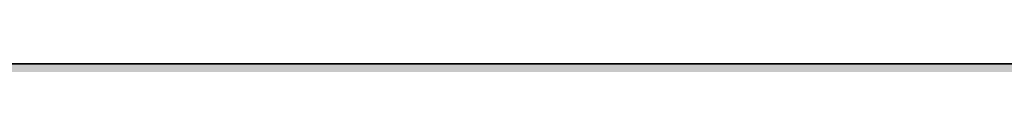
# Model space of a CAD drawing. Units: inches. Extents: x 2091 to 2899, y 967 to 2217.
# Tile 100 of 256: x 2252.3817 to 2252.951, y 1099.9191 to 1099.9191. Entities that reach past the tile are written whole.
import ezdxf

# ---------------------------------------------------------------- set-up
doc = ezdxf.new("R2010")
doc.units = ezdxf.units.IN
doc.layers.add('A-WALL-PATT', color=141, linetype='Continuous', lineweight=13, true_color=0xadddf7)
doc.layers.add('L-SITE-WALL', color=7, linetype='Continuous', lineweight=35)

msp = doc.modelspace()

# ---------------------------------------------------------------- hatches: boundary and pattern name
at = {"layer": 'A-WALL-PATT'}
h = msp.add_hatch(color=256, dxfattribs=at)
h.dxf.hatch_style = 1
h.paths.add_polyline_path([(2212.1436, 1941.41906), (2387.6436, 1941.41906), (2387.6436, 1824.41906), (2392.1436, 1824.41906), (2392.1436, 1941.41906), (2609.6436, 1941.41906), (2609.6436, 1825.91906), (2614.1436, 1825.91906), (2614.1436, 1941.41906), (2794.1436, 1941.41906), (2794.1436, 1928.76217), (2803.1436, 1928.76217), (2803.1436, 2050.91906), (2203.1436, 2050.91906), (2203.1436, 1900.75786), (2212.1436, 1900.75786)])
h.paths.add_polyline_path([(2212.1436, 1945.91906), (2212.1436, 2041.91906), (2794.1436, 2041.91906), (2794.1436, 1945.91906), (2402.24824, 1945.91906), (2401.10243, 1945.77583), (2398.70243, 1945.77583)], flags=16)
h.paths.add_polyline_path([(2230.22986, 1948.06279), (2227.34986, 1949.50279), (2225.90986, 1951.90279), (2223.98986, 1952.86279), (2223.02986, 1955.26279), (2222.06986, 1959.58279), (2222.06986, 1963.42279), (2223.02986, 1965.66279), (2223.98986, 1965.34279), (2225.58591, 1963.86075), (2226.91153, 1964.95726), (2226.94886, 1965.93879), (2227.77832, 1966.95214), (2228.19992, 1968.8787), (2230.70986, 1964.86279), (2233.58986, 1966.30279), (2233.60731, 1966.33187), (2233.77266, 1964.9382), (2234.6338, 1963.67647), (2235.02986, 1963.90279), (2236.28203, 1965.57236), (2235.98986, 1962.94279), (2237.95451, 1957.54), (2238.38986, 1957.90279), (2239.21586, 1960.30579), (2238.65457, 1966.38496), (2238.69279, 1966.43807), (2238.84058, 1967.49971), (2238.78029, 1967.68749), (2238.88054, 1967.78676), (2238.66686, 1966.25179), (2239.21586, 1960.30579), (2238.38986, 1957.90279), (2236.94986, 1956.70279), (2234.54986, 1949.98279)], flags=0)
h.paths.add_polyline_path([(2278.01197, 1948.06279), (2276.49643, 1947.87335), (2275.84983, 1947.68861), (2274.65197, 1947.10279)], flags=0)
h.paths.add_polyline_path([(2269.85197, 1955.74279), (2268.27618, 1956.62933), (2270.8673, 1956.3484), (2269.37197, 1958.14279), (2268.71496, 1959.19233), (2270.56983, 1958.72861), (2268.58073, 1961.90609), (2270.81197, 1960.89188), (2270.81197, 1963.42279), (2271.39331, 1964.77926), (2270.29176, 1966.1562), (2271.77197, 1965.66279), (2272.14139, 1966.52476), (2273.92983, 1965.92861), (2275.63039, 1968.0543), (2276.33194, 1966.72186), (2276.52043, 1966.95214), (2276.94203, 1968.8787), (2277.73429, 1967.61108), (2278.13989, 1969.46452), (2279.65912, 1967.03374), (2280.41197, 1966.78279), (2280.9493, 1967.58879), (2281.60983, 1967.36861), (2282.13327, 1968.15376), (2282.34924, 1966.33344), (2282.34985, 1966.33259), (2283.40755, 1968.09542), (2283.71263, 1965.52402), (2284.32022, 1964.63379), (2284.51181, 1964.88924), (2284.23497, 1965.70479), (2284.50047, 1967.31896), (2284.90794, 1965.41742), (2285.39631, 1966.06858), (2285.43283, 1966.29061), (2285.47334, 1966.17128), (2286.35392, 1967.34539), (2286.22201, 1966.15817), (2287.66349, 1968.08015), (2287.71397, 1968.44279), (2288.4816, 1969.01668), (2288.57399, 1968.7289), (2288.91746, 1969.06904), (2288.60683, 1966.83761), (2288.92873, 1963.35131), (2288.93497, 1963.35679), (2288.92973, 1963.34042), (2289.01528, 1962.41387), (2290.11122, 1963.87513), (2290.13283, 1963.94261), (2290.21767, 1964.01706), (2290.11122, 1963.87513), (2289.15583, 1960.89161), (2288.59404, 1959.25723), (2288.57197, 1959.10279), (2289.53197, 1960.54279), (2290.01197, 1962.46279), (2290.19184, 1962.64266), (2289.76983, 1959.68861), (2286.88983, 1957.28861), (2284.48983, 1950.56861), (2283.31466, 1950.04631), (2283.29197, 1949.98279), (2280.29006, 1948.64861), (2281.12983, 1948.64861), (2282.56983, 1948.16861), (2283.20473, 1948.06279), (2278.97197, 1948.06279), (2276.09197, 1949.50279), (2274.65197, 1951.90279), (2272.73197, 1952.86279)], flags=0)
h.paths.add_polyline_path([(2271.15887, 1958.02177), (2272.96983, 1955.84861), (2272.00983, 1960.16861), (2272.00983, 1964.00861), (2272.62443, 1965.44266), (2274.32802, 1963.86075), (2275.65365, 1964.95726), (2275.63774, 1964.53909), (2277.41223, 1966.00689), (2277.03297, 1965.15679), (2276.82992, 1964.9756), (2276.76601, 1963.29501), (2277.44964, 1962.66022), (2279.45197, 1964.86279), (2282.33197, 1966.30279), (2283.52983, 1966.88861), (2283.29451, 1966.77095), (2283.91299, 1963.8847), (2284.89925, 1964.44827), (2284.73197, 1962.94279), (2286.69662, 1957.54), (2287.13197, 1957.90279), (2287.54191, 1959.09539), (2287.7794, 1958.44231), (2285.68274, 1956.6951), (2285.8765, 1959.79534), (2284.73197, 1962.94279), (2284.89925, 1964.44827), (2283.91299, 1963.8847), (2284.22383, 1962.43412), (2283.42436, 1963.60548), (2281.60983, 1962.56861), (2281.12983, 1960.16861), (2282.08983, 1956.32861), (2283.04983, 1952.96861), (2282.56983, 1950.56861), (2280.16983, 1948.64861), (2279.88332, 1948.79187), (2278.97197, 1948.06279), (2278.97197, 1949.02279), (2278.67231, 1949.39737), (2277.28983, 1950.08861), (2275.84983, 1952.48861), (2273.92983, 1953.44861), (2272.48983, 1954.88861), (2271.92165, 1954.88861), (2271.77197, 1955.26279)], flags=0)
h.paths.add_polyline_path([(2311.99415, 1955.74279), (2312.06272, 1955.67422), (2312.0551, 1955.7085)], flags=0)
h.paths.add_polyline_path([(2331.95615, 1963.95179), (2333.39615, 1965.39179), (2331.07715, 1963.35679), (2330.9986, 1963.11152)], flags=0)
h.paths.add_polyline_path([(2310.55415, 1954.30279), (2307.03981, 1956.27994), (2310.7629, 1955.87628), (2312.47415, 1953.82279), (2313.43415, 1951.42279), (2315.35415, 1950.46279), (2316.79415, 1948.06279), (2317.46615, 1947.72679), (2319.36869, 1947.96461), (2317.75415, 1949.98279), (2317.56953, 1950.61048), (2316.79415, 1951.90279), (2314.87415, 1952.86279), (2313.91415, 1955.26279), (2311.51415, 1958.14279), (2309.37549, 1961.55917), (2311.51415, 1960.33708), (2311.51415, 1961.98279), (2310.60467, 1963.11963), (2311.72661, 1962.47853), (2312.41833, 1964.09256), (2312.25596, 1964.29552), (2313.19415, 1963.98279), (2313.91415, 1965.66279), (2314.64678, 1965.41858), (2315.35415, 1966.30279), (2316.79415, 1967.74279), (2316.15744, 1966.9469), (2317.03411, 1965.28186), (2317.2226, 1965.51214), (2317.77705, 1968.04577), (2318.47411, 1966.72186), (2318.6626, 1966.95214), (2319.0842, 1968.8787), (2321.20705, 1965.48215), (2322.16142, 1966.9137), (2322.55415, 1966.78279), (2322.78599, 1967.13056), (2322.88165, 1966.32429), (2323.31204, 1965.72174), (2323.65129, 1965.89136), (2324.3965, 1967.13338), (2324.65694, 1964.9382), (2324.97199, 1964.47661), (2325.38728, 1967.0015), (2325.94081, 1964.41835), (2327.22893, 1966.13584), (2327.16632, 1965.57236), (2328.05914, 1966.76278), (2328.22458, 1966.24749), (2329.66797, 1967.67691), (2329.66458, 1967.68749), (2329.76482, 1967.78676), (2329.55115, 1966.25179), (2330.10015, 1960.30579), (2329.33281, 1958.07347), (2329.31306, 1957.93523), (2329.63415, 1958.20279), (2330.23415, 1959.10279), (2330.71415, 1961.02279), (2331.03415, 1961.34279), (2330.71415, 1959.10279), (2329.63415, 1958.20279), (2329.27415, 1957.66279), (2327.71211, 1956.3611), (2325.43415, 1949.98279), (2324.33377, 1949.49374), (2323.99415, 1948.54279), (2319.67415, 1946.62279), (2316.79415, 1948.06279), (2315.35415, 1950.46279), (2313.43415, 1951.42279)], flags=0)
h.paths.add_polyline_path([(2321.33568, 1947.95202), (2321.11415, 1948.06279), (2321.11415, 1949.02279), (2319.19415, 1951.42279), (2316.79415, 1959.58279), (2316.66324, 1959.58279), (2315.35415, 1958.14279), (2314.39415, 1958.14279), (2313.1483, 1958.70908), (2312.95415, 1959.58279), (2312.95415, 1960.89188), (2315.83415, 1959.58279), (2316.66324, 1959.58279), (2317.31471, 1960.29941), (2315.0302, 1962.42075), (2316.35582, 1963.51726), (2316.37234, 1963.95162), (2316.4702, 1963.86075), (2317.79582, 1964.95726), (2317.75522, 1963.88969), (2319.17515, 1965.15679), (2319.49841, 1965.88137), (2321.11415, 1965.34279), (2323.23589, 1962.37236), (2325.68635, 1963.77262), (2325.54279, 1962.48058), (2325.19878, 1963.49401), (2324.47851, 1963.08243), (2324.92601, 1960.99412), (2324.07809, 1962.23647), (2322.41479, 1961.28602), (2322.07415, 1959.58279), (2323.03415, 1955.74279), (2323.99415, 1952.38279), (2323.51415, 1949.98279), (2322.14272, 1948.88565), (2322.07415, 1948.54279)], flags=0)
h.paths.add_polyline_path([(2320.20748, 1963.33746), (2320.15415, 1963.42279), (2320.39415, 1963.54279)], flags=0)
h.paths.add_polyline_path([(2353.85053, 1965.8105), (2354.03053, 1965.7505), (2354.33053, 1966.4505), (2354.33053, 1966.9305)], flags=0)
h.paths.add_polyline_path([(2359.02058, 1969.02641), (2359.09838, 1968.90193), (2359.23353, 1969.5195), (2359.23353, 1969.9995)], flags=0)
h.paths.add_polyline_path([(2358.25669, 1966.68167), (2357.9836, 1966.34803), (2358.21127, 1966.14617), (2358.41049, 1966.38957)], flags=0)
h.paths.add_polyline_path([(2357.76847, 1966.05878), (2357.7322, 1965.10497), (2357.75105, 1965.12056), (2357.76953, 1965.6065), (2357.76953, 1966.05784)], flags=0)
h.paths.add_polyline_path([(2359.11153, 1965.3045), (2359.11153, 1964.8245), (2359.84453, 1966.4675), (2359.84453, 1966.9475)], flags=0)
h.paths.add_polyline_path([(2360.22368, 1966.62145), (2360.69853, 1969.3625), (2360.69853, 1969.8425), (2360.21053, 1967.0255), (2360.21053, 1966.6425)], flags=0)
h.paths.add_polyline_path([(2363.45053, 1967.8905), (2363.45053, 1968.3705), (2362.49053, 1966.9305), (2362.65604, 1966.69878)], flags=0)
h.paths.add_polyline_path([(2364.47552, 1966.07883), (2365.85053, 1968.3705), (2365.85053, 1968.8505), (2364.42798, 1966.47958)], flags=0)
h.paths.add_polyline_path([(2366.31353, 1965.8525), (2366.36671, 1965.69583), (2366.80253, 1968.3455), (2366.80253, 1968.8255)], flags=0)
h.paths.add_polyline_path([(2367.16531, 1965.80354), (2367.29053, 1966.9305), (2367.29053, 1967.4105), (2367.1027, 1965.72007)], flags=0)
h.paths.add_polyline_path([(2370.03653, 1959.9735), (2371.01353, 1963.0245), (2371.01353, 1963.5045), (2370.03653, 1960.4535)], flags=0)
h.paths.add_polyline_path([(2371.61053, 1960.2105), (2372.57053, 1961.6505), (2372.57053, 1962.1305), (2371.80253, 1960.9785)], flags=0)
h.paths.add_polyline_path([(2350.87367, 1956.00509), (2351.93053, 1955.8905), (2354.49053, 1953.3305), (2353.85053, 1954.9305), (2351.45053, 1957.8105), (2347.93553, 1963.4255), (2347.93553, 1963.9055), (2351.45053, 1958.2905), (2353.70507, 1955.58505), (2352.89053, 1959.2505), (2352.89053, 1959.7305), (2352.89053, 1961.92479), (2356.73053, 1959.7305), (2358.45447, 1961.62684), (2354.81053, 1965.0105), (2355.03086, 1965.28591), (2358.69109, 1961.88712), (2361.53053, 1965.0105), (2364.3765, 1966.43348), (2364.52439, 1965.18691), (2365.45447, 1963.82418), (2365.88107, 1964.06795), (2365.37053, 1966.4505), (2365.37053, 1966.9305), (2366.81053, 1960.2105), (2366.81053, 1959.7305), (2366.38871, 1952.98141), (2367.77053, 1956.8505), (2368.64123, 1957.57608), (2366.81053, 1962.6105), (2366.81053, 1963.0905), (2368.77518, 1957.68771), (2369.21053, 1958.0505), (2370.00159, 1960.35187), (2369.47523, 1966.05267), (2369.51346, 1966.10578), (2369.51417, 1966.11091), (2369.47523, 1966.53267), (2369.51346, 1966.58578), (2369.61463, 1967.31259), (2369.18253, 1968.6585), (2369.18253, 1969.1385), (2369.60096, 1967.83519), (2369.7012, 1967.93447), (2369.71795, 1968.05474), (2370.14518, 1968.37414), (2369.77871, 1968.01122), (2369.7012, 1967.45447), (2370.46816, 1968.214), (2369.67494, 1967.26577), (2369.51417, 1966.11091), (2370.03653, 1960.4535), (2370.03653, 1959.9735), (2369.44176, 1958.24319), (2370.65053, 1959.2505), (2371.04582, 1962.01756), (2371.13053, 1962.1305), (2370.65053, 1958.7705), (2367.77053, 1956.3705), (2365.37053, 1949.6505), (2362.0791, 1948.18764), (2363.45053, 1947.7305), (2361.05053, 1947.7305), (2360.09053, 1947.7305), (2357.10386, 1947.35717), (2360.09053, 1948.2105), (2358.17053, 1949.1705), (2356.73053, 1951.5705), (2354.81053, 1952.5305), (2351.93053, 1955.4105)], flags=0)
h.paths.add_polyline_path([(2361.05053, 1948.6905), (2359.13053, 1951.0905), (2356.73053, 1959.2505), (2355.77053, 1959.2505), (2352.89053, 1960.55959), (2352.89053, 1961.44479), (2355.89053, 1959.7305), (2356.73053, 1959.7305), (2356.83719, 1959.36783), (2361.53053, 1964.5305), (2363.24842, 1965.38945), (2364.92531, 1963.0418), (2362.49053, 1961.6505), (2362.06386, 1959.51717), (2362.97053, 1955.8905), (2363.93053, 1952.5305), (2363.93053, 1952.0505), (2363.45053, 1949.6505), (2361.05053, 1947.7305)], flags=0)
h.paths.add_polyline_path([(2359.13053, 1951.5705), (2359.29053, 1951.3705), (2361.05053, 1954.4505), (2361.05053, 1954.9305)], flags=0)
h.paths.add_polyline_path([(2357.21953, 1966.5455), (2356.79253, 1968.8145), (2356.79253, 1969.2945), (2357.21953, 1967.0255)], flags=0)
h.paths.add_polyline_path([(2361.05053, 1954.4505), (2361.53053, 1958.7705), (2361.53053, 1959.2505), (2361.05053, 1954.9305)], flags=0)
h.paths.add_polyline_path([(2402.54829, 1948.48608), (2402.30243, 1948.41583), (2402.59043, 1948.41583)], flags=0)
h.paths.add_polyline_path([(2394.14243, 1956.09583), (2395.68505, 1954.55321), (2396.7205, 1953.97068), (2396.06243, 1955.61583), (2395.24138, 1956.6011), (2395.8789, 1956.44171), (2395.10243, 1959.93583), (2395.10243, 1963.77583), (2396.06243, 1966.01583), (2397.02243, 1965.69583), (2398.61848, 1964.21379), (2399.94411, 1965.3103), (2399.98143, 1966.29183), (2400.81089, 1967.30518), (2401.23249, 1969.23174), (2403.53795, 1965.54301), (2403.94198, 1967.38932), (2404.70243, 1967.13583), (2405.46033, 1966.07478), (2406.62243, 1966.65583), (2406.63988, 1966.68491), (2406.80523, 1965.29124), (2406.92569, 1965.11475), (2407.34243, 1964.97583), (2407.87433, 1965.77367), (2408.1691, 1964.39805), (2409.31461, 1965.9254), (2409.21746, 1965.05105), (2409.44523, 1963.13124), (2410.30637, 1961.86951), (2410.70243, 1962.09583), (2411.44227, 1963.08228), (2411.16543, 1963.89783), (2411.61643, 1966.63976), (2411.72536, 1966.79111), (2411.87315, 1967.85275), (2411.81286, 1968.04053), (2411.91311, 1968.1398), (2411.69943, 1966.60483), (2412.24843, 1960.65883), (2413.22543, 1963.70983), (2414.3779, 1964.72116), (2414.51315, 1965.69275), (2414.45286, 1965.88053), (2414.55311, 1965.9798), (2414.3779, 1964.72116), (2414.51982, 1964.8457), (2414.36536, 1964.63111), (2414.33943, 1964.44483), (2414.88843, 1958.49883), (2414.06243, 1956.09583), (2412.62243, 1954.89583), (2410.17137, 1948.03285), (2410.01672, 1948.0844), (2405.90243, 1946.25583), (2405.90243, 1947.21583), (2405.20425, 1948.08856), (2404.22243, 1948.41583), (2403.26243, 1948.41583), (2400.38243, 1949.85583), (2399.66243, 1951.05583), (2397.98243, 1952.73583), (2397.02243, 1953.21583), (2395.68505, 1954.55321), (2392.65678, 1956.25691)], flags=0)
h.paths.add_polyline_path([(2409.08565, 1964.40744), (2409.13036, 1964.27572), (2409.26243, 1964.49583)], flags=0)
h.paths.add_polyline_path([(2397.74243, 1961.61583), (2398.70243, 1963.85583), (2399.66243, 1963.53583), (2401.42656, 1965.74099), (2401.79142, 1966.5588), (2402.07143, 1965.07083), (2402.83551, 1964.39337), (2403.2624, 1964.9149), (2403.33812, 1964.77109), (2402.61552, 1963.97622), (2402.49861, 1960.90224), (2403.543, 1959.93245), (2404.4132, 1960.88968), (2404.70243, 1962.33583), (2407.91635, 1964.17235), (2409.52021, 1961.92694), (2410.98708, 1957.89304), (2411.42243, 1958.25583), (2412.04796, 1960.07562), (2412.41034, 1959.07909), (2411.67562, 1958.46682), (2411.66243, 1958.25583), (2411.62607, 1958.42553), (2409.98243, 1957.05583), (2407.58243, 1950.33583), (2403.26243, 1948.41583), (2403.26243, 1949.37583), (2401.34243, 1951.77583), (2399.41651, 1958.32398), (2397.74243, 1959.08492), (2397.74243, 1959.97012), (2397.10243, 1960.33583), (2397.74243, 1960.04492)], flags=0)
h.paths.add_polyline_path([(2405.90243, 1952.97583), (2405.95043, 1953.40783), (2406.01672, 1953.17583)], flags=0)
h.paths.add_polyline_path([(2449.81778, 1967.11401), (2449.75232, 1967.13583), (2449.7937, 1967.0779)], flags=0)
h.paths.add_polyline_path([(2451.6977, 1966.61812), (2451.74089, 1966.69012), (2451.69205, 1966.6657)], flags=0)
h.paths.add_polyline_path([(2454.34363, 1965.73757), (2455.75232, 1967.61583), (2455.99232, 1968.09583), (2454.3645, 1965.9254)], flags=0)
h.paths.add_polyline_path([(2457.54732, 1968.86383), (2457.78732, 1969.34383), (2457.05432, 1968.79583), (2457.00762, 1968.46034)], flags=0)
h.paths.add_polyline_path([(2456.92178, 1967.85666), (2456.80224, 1968.22902), (2456.723, 1967.6598)], flags=0)
h.paths.add_polyline_path([(2457.30232, 1967.37683), (2457.54232, 1967.85683), (2456.81032, 1966.83983), (2456.74052, 1966.70022), (2456.74902, 1966.60811)], flags=0)
h.paths.add_polyline_path([(2458.27532, 1963.70983), (2458.15534, 1963.33515), (2460.35432, 1965.26483), (2460.59432, 1965.74483)], flags=0)
h.paths.add_polyline_path([(2458.39232, 1962.81583), (2458.36409, 1962.61819), (2459.59232, 1964.25583), (2459.83232, 1964.73583)], flags=0)
h.paths.add_polyline_path([(2459.35232, 1962.81583), (2459.27232, 1962.49583), (2460.07232, 1963.29583), (2460.31232, 1963.77583)], flags=0)
h.paths.add_polyline_path([(2458.68032, 1960.60783), (2458.63232, 1960.41583), (2459.59232, 1961.85583), (2459.83232, 1962.33583)], flags=0)
h.paths.add_polyline_path([(2437.83817, 1956.24265), (2439.19232, 1956.09583), (2441.35232, 1953.93583), (2440.87232, 1955.13583), (2438.47232, 1958.01583), (2438.07156, 1958.65602), (2438.71232, 1958.49583), (2440.6396, 1956.18311), (2439.91232, 1959.45583), (2439.91232, 1963.29583), (2441.35232, 1966.65583), (2441.59232, 1967.13583), (2441.11232, 1966.01583), (2442.07232, 1965.69583), (2443.98899, 1968.09167), (2444.24132, 1966.75083), (2444.9168, 1966.15192), (2445.67657, 1967.08014), (2446.25532, 1969.72483), (2446.49532, 1970.20483), (2446.28238, 1969.23174), (2447.36267, 1967.50327), (2447.72032, 1969.56783), (2447.96032, 1970.04783), (2447.48548, 1967.30678), (2448.79232, 1965.21583), (2448.47232, 1964.86383), (2448.55232, 1964.73583), (2451.45205, 1966.1857), (2451.61512, 1964.81124), (2452.30792, 1963.79617), (2453.23451, 1964.32565), (2454.07232, 1960.41583), (2453.62869, 1953.31765), (2454.79232, 1956.57583), (2455.03232, 1957.05583), (2455.71884, 1957.62793), (2453.83232, 1962.81583), (2453.94097, 1963.79362), (2453.33532, 1965.57783), (2453.82432, 1968.55083), (2454.06432, 1969.03083), (2453.57532, 1966.05783), (2454.04033, 1964.68792), (2453.83232, 1962.81583), (2455.71884, 1957.62793), (2456.36721, 1958.16824), (2457.05832, 1960.17883), (2457.29832, 1960.65883), (2456.47232, 1958.25583), (2457.71773, 1959.29367), (2457.67232, 1958.97583), (2454.88995, 1956.65719), (2453.61414, 1953.08492), (2453.59232, 1952.73583), (2453.35232, 1952.25583), (2453.3596, 1952.3722), (2452.63232, 1950.33583), (2452.39232, 1949.85583), (2449.20375, 1948.43869), (2450.71232, 1947.93583), (2448.07232, 1947.93583), (2447.11232, 1947.93583), (2444.55232, 1947.61583), (2447.1996, 1948.3722), (2445.19232, 1949.37583), (2443.75232, 1951.77583), (2441.83232, 1952.73583), (2438.95232, 1955.61583)], flags=0)
h.paths.add_polyline_path([(2443.99232, 1959.93583), (2444.04032, 1959.77263), (2444.12155, 1959.86199)], flags=0)
h.paths.add_polyline_path([(2442.91232, 1959.93583), (2443.03232, 1959.93583), (2442.44566, 1960.2025)], flags=0)
h.paths.add_polyline_path([(2444.98294, 1965.01968), (2445.27932, 1965.26483), (2445.51932, 1965.74483), (2444.994, 1965.3103)], flags=0)
h.paths.add_polyline_path([(2446.13332, 1965.02983), (2446.33037, 1965.4715), (2444.97032, 1964.25783), (2444.73032, 1963.77783)], flags=0)
h.paths.add_polyline_path([(2442.79232, 1959.45583), (2443.75232, 1959.45583), (2446.15232, 1951.29583), (2446.41232, 1951.75083), (2446.39232, 1951.77583), (2448.0806, 1954.73032), (2448.55232, 1958.97583), (2441.83232, 1965.21583), (2442.15495, 1965.61911), (2448.79232, 1959.45583), (2448.31232, 1955.13583), (2448.07232, 1954.65583), (2446.41232, 1951.75083), (2448.31232, 1949.37583), (2448.31232, 1948.41583), (2450.54089, 1950.19869), (2450.95232, 1952.25583), (2449.99232, 1955.61583), (2449.03232, 1959.45583), (2449.51232, 1961.85583), (2449.75232, 1962.33583), (2449.6749, 1961.94874), (2452.99451, 1963.84565), (2453.06441, 1963.51941), (2452.88461, 1963.78285), (2449.6749, 1961.94874), (2449.27232, 1959.93583), (2450.23232, 1956.09583), (2451.19232, 1952.73583), (2450.71232, 1950.33583), (2450.47232, 1949.85583), (2448.07232, 1947.93583), (2448.07232, 1948.53583), (2445.43232, 1949.85583), (2443.99232, 1952.25583), (2442.07232, 1953.21583), (2441.11232, 1955.61583), (2440.15232, 1959.93583), (2440.15232, 1960.65583)], flags=0)
h.paths.add_polyline_path([(2456.69232, 1966.98583), (2457.60832, 1968.08083), (2457.84832, 1968.56083), (2456.93232, 1967.46583)], flags=0)
h.paths.add_polyline_path([(2489.89657, 1966.58024), (2489.94295, 1966.18935), (2490.74749, 1967.53025), (2491.31912, 1968.95116)], flags=0)
h.paths.add_polyline_path([(2473.56247, 1956.40713), (2477.13998, 1956.01926), (2476.95533, 1956.24083), (2475.10805, 1957.28011), (2476.34749, 1956.97025), (2475.1869, 1958.82422), (2476.91912, 1958.39116), (2475.41164, 1960.79927), (2477.78749, 1959.71934), (2477.78749, 1962.25025), (2477.6374, 1962.43786), (2477.82255, 1962.33206), (2478.35912, 1963.58406), (2478.35912, 1963.67116), (2477.32435, 1964.96463), (2478.71483, 1964.50114), (2479.31912, 1965.91116), (2480.27912, 1965.59116), (2481.78397, 1967.47221), (2482.11649, 1965.70525), (2482.88056, 1965.02778), (2483.20931, 1965.42941), (2483.22017, 1965.71509), (2483.07594, 1965.98902), (2483.71176, 1966.76581), (2484.13049, 1968.67925), (2484.70212, 1970.10016), (2484.48918, 1969.12707), (2486.5029, 1965.90511), (2487.38749, 1965.61025), (2488.15342, 1966.75914), (2488.71702, 1965.97011), (2489.20009, 1966.21164), (2489.33067, 1965.11099), (2490.3939, 1963.62246), (2490.66077, 1963.77496), (2490.49391, 1964.55364), (2490.92306, 1963.92484), (2491.31912, 1964.15116), (2491.33339, 1964.17018), (2491.21049, 1964.53225), (2491.28176, 1964.96554), (2491.42579, 1964.29338), (2494.07648, 1967.82763), (2494.49792, 1966.51494), (2494.59817, 1966.61422), (2494.68949, 1967.27025), (2495.10675, 1967.5822), (2495.12984, 1967.74807), (2495.06955, 1967.93585), (2495.1698, 1968.03513), (2495.03178, 1967.04363), (2495.75382, 1967.75868), (2494.98205, 1966.68644), (2494.95612, 1966.50016), (2495.47902, 1960.83685), (2495.91049, 1962.18425), (2496.48212, 1963.60516), (2496.07269, 1962.32659), (2496.7689, 1962.93754), (2496.59912, 1962.71116), (2496.11912, 1959.35116), (2496.73287, 1960.27179), (2496.98749, 1961.29025), (2497.55912, 1962.71116), (2497.07912, 1960.79116), (2496.50749, 1959.37025), (2495.54749, 1957.93025), (2492.75884, 1955.60638), (2490.83912, 1950.23116), (2490.26749, 1948.81025), (2485.94749, 1946.89025), (2483.06749, 1948.33025), (2481.62749, 1950.73025), (2479.70749, 1951.69025), (2476.82749, 1954.57025)], flags=0)
h.paths.add_polyline_path([(2485.57697, 1948.31339), (2485.55912, 1948.31116), (2485.57876, 1948.31116)], flags=0)
h.paths.add_polyline_path([(2478.64506, 1954.55116), (2478.10904, 1956.96326), (2479.31912, 1955.51116), (2480.27912, 1953.11116), (2482.19912, 1952.15116), (2483.63912, 1949.75116), (2486.51912, 1948.31116), (2486.51912, 1949.27116), (2484.73931, 1951.49593), (2484.02749, 1950.25025), (2481.62749, 1958.41025), (2482.37515, 1959.23267), (2482.19912, 1959.83116), (2483.19757, 1960.92946), (2479.70749, 1964.17025), (2480.60336, 1965.29008), (2481.87517, 1964.10911), (2482.66639, 1964.76358), (2482.61536, 1963.4218), (2482.9892, 1963.07466), (2484.00849, 1963.98425), (2484.68361, 1965.49751), (2484.58012, 1965.40516), (2485.35727, 1967.14711), (2485.12065, 1965.7812), (2486.42749, 1963.69025), (2488.14538, 1964.5492), (2489.82227, 1962.20155), (2490.74749, 1962.73025), (2491.99966, 1964.39981), (2492.07605, 1965.08726), (2492.21289, 1964.68412), (2492.48537, 1965.04743), (2492.27912, 1963.19116), (2494.24377, 1957.78837), (2494.5625, 1958.05398), (2494.93349, 1959.13325), (2495.50512, 1960.55416), (2494.67912, 1958.15116), (2494.10749, 1956.73025), (2494.5625, 1958.05398), (2493.40854, 1957.09235), (2491.70749, 1961.77025), (2491.99966, 1964.39981), (2490.74749, 1962.73025), (2487.71203, 1960.9957), (2487.47912, 1959.83116), (2488.43912, 1955.99116), (2489.39912, 1952.63116), (2488.91912, 1950.23116), (2488.57692, 1949.9574), (2488.34749, 1948.81025), (2487.65172, 1948.25363), (2487.47912, 1948.31116), (2486.51912, 1948.31116), (2483.63912, 1949.75116), (2482.19912, 1952.15116), (2480.27912, 1953.11116), (2478.83912, 1954.55116)], flags=0)
h.paths.add_polyline_path([(2526.64825, 1966.98752), (2526.51734, 1967.03116), (2526.6001, 1966.9153)], flags=0)
h.paths.add_polyline_path([(2528.47064, 1966.44666), (2528.57449, 1966.61973), (2528.45707, 1966.56102)], flags=0)
h.paths.add_polyline_path([(2534.13334, 1967.49616), (2534.15669, 1967.54285), (2534.05984, 1967.4083)], flags=0)
h.paths.add_polyline_path([(2536.16192, 1964.0506), (2535.15734, 1962.71116), (2535.10087, 1962.31587), (2536.11734, 1963.67116), (2536.42053, 1964.27754)], flags=0)
h.paths.add_polyline_path([(2535.15734, 1959.83116), (2536.11734, 1961.27116), (2536.59734, 1962.23116), (2535.25334, 1960.21516)], flags=0)
h.paths.add_polyline_path([(2513.24904, 1956.2848), (2516.22118, 1955.96256), (2514.99734, 1957.43116), (2514.19582, 1958.71154), (2515.47734, 1958.39116), (2516.93189, 1956.64571), (2516.43734, 1958.87116), (2516.43734, 1962.71116), (2516.87269, 1963.72697), (2515.34643, 1965.6348), (2517.39734, 1964.95116), (2517.87734, 1966.07116), (2518.35734, 1967.03116), (2517.87734, 1965.91116), (2518.83734, 1965.59116), (2520.48659, 1967.65272), (2520.76634, 1966.16616), (2521.53042, 1965.48869), (2521.78144, 1965.79537), (2521.80091, 1966.30727), (2521.4778, 1966.92094), (2521.24634, 1967.12616), (2521.1777, 1967.49091), (2521.4778, 1966.92094), (2522.01042, 1966.44869), (2522.25739, 1966.75042), (2522.78034, 1969.14016), (2523.26034, 1970.10016), (2523.0474, 1969.12707), (2524.67313, 1966.5259), (2526.03734, 1966.07116), (2526.79524, 1965.01011), (2527.97707, 1965.60102), (2528.14014, 1964.22657), (2528.66459, 1963.45816), (2529.38862, 1963.87189), (2529.32967, 1964.14699), (2529.48128, 1963.92484), (2529.87734, 1964.15116), (2529.98401, 1964.29338), (2529.78905, 1965.20318), (2530.0624, 1964.3979), (2532.80248, 1968.05135), (2533.14777, 1966.97585), (2533.24802, 1967.07513), (2533.33934, 1967.73116), (2533.67285, 1967.98049), (2533.72802, 1968.03513), (2533.51434, 1966.50016), (2534.02472, 1960.9725), (2534.56034, 1962.64516), (2535.04034, 1963.60516), (2534.06334, 1960.55416), (2533.23734, 1958.15116), (2534.28815, 1959.02684), (2534.19734, 1958.39116), (2531.5126, 1956.15387), (2529.39734, 1950.23116), (2528.91734, 1949.27116), (2526.44877, 1948.17402), (2527.47734, 1947.83116), (2530.35734, 1947.35116), (2524.59734, 1947.35116), (2521.71734, 1948.79116), (2520.27734, 1951.19116), (2518.35734, 1952.15116), (2515.47734, 1955.03116)], flags=0)
h.paths.add_polyline_path([(2523.93476, 1967.19031), (2523.61951, 1966.48369), (2523.7705, 1966.24211)], flags=0)
h.paths.add_polyline_path([(2518.83734, 1953.11116), (2517.87734, 1955.51116), (2516.88498, 1959.97678), (2516.91734, 1959.96207), (2516.91734, 1962.02545), (2520.75734, 1959.83116), (2522.02495, 1961.22553), (2518.35734, 1964.63116), (2519.00259, 1965.43772), (2520.43339, 1964.10911), (2521.30112, 1964.82687), (2521.24516, 1963.35533), (2525.63831, 1959.27598), (2526.03734, 1961.27116), (2529.39734, 1963.19116), (2530.64952, 1964.86073), (2530.66472, 1964.99755), (2530.69196, 1964.91731), (2531.08778, 1965.44507), (2530.94599, 1964.16894), (2530.69196, 1964.91731), (2529.39734, 1963.19116), (2526.3625, 1961.45697), (2526.03734, 1959.83116), (2526.99734, 1955.99116), (2527.95734, 1952.63116), (2527.47734, 1950.23116), (2527.13449, 1949.95687), (2526.97393, 1949.15409), (2526.69734, 1949.03116), (2524.59734, 1947.35116), (2524.59734, 1948.31116), (2524.27734, 1948.71116), (2522.19734, 1949.75116), (2520.75734, 1952.15116)], flags=0)
h.paths.add_polyline_path([(2520.27734, 1958.87116), (2520.85334, 1959.50476), (2523.15734, 1951.67116), (2524.61389, 1954.22013), (2524.59734, 1954.07116), (2522.67734, 1950.71116)], flags=0)
h.paths.add_polyline_path([(2559.37091, 1966.31116), (2559.39841, 1966.32491), (2559.40194, 1966.3453)], flags=0)
h.paths.add_polyline_path([(2549.77091, 1957.19116), (2552.65091, 1954.31116), (2552.13399, 1955.60347), (2550.61091, 1957.43116), (2547.09591, 1963.04616), (2545.77591, 1965.20616), (2549.29091, 1959.59116), (2551.69091, 1956.71116), (2550.79293, 1960.75206), (2550.73091, 1960.78025), (2550.73091, 1964.87116), (2551.69091, 1967.11116), (2552.65091, 1966.79116), (2554.24696, 1965.30911), (2555.03425, 1965.96034), (2555.58167, 1966.64461), (2555.60991, 1967.38716), (2556.43937, 1968.40051), (2556.86097, 1970.32707), (2559.37091, 1966.31116), (2560.69091, 1964.15116), (2562.40881, 1965.01011), (2561.65091, 1966.07116), (2560.33091, 1968.23116), (2561.7585, 1966.23254), (2562.34721, 1967.11561), (2562.43371, 1966.38657), (2563.1278, 1965.3696), (2563.57091, 1965.59116), (2563.58836, 1965.62024), (2563.36254, 1967.52354), (2563.72249, 1965.84379), (2565.06, 1968.07298), (2564.73286, 1965.12872), (2565.11758, 1963.33338), (2567.44462, 1966.43611), (2567.31561, 1967.83333), (2567.35384, 1967.88644), (2567.50163, 1968.94807), (2567.44134, 1969.13585), (2567.54159, 1969.23513), (2567.32791, 1967.70016), (2567.87691, 1961.75416), (2568.74669, 1964.47033), (2568.63561, 1965.67333), (2568.67384, 1965.72644), (2568.82163, 1966.78807), (2568.76134, 1966.97585), (2568.86159, 1967.07513), (2568.64791, 1965.54016), (2568.72613, 1964.69303), (2568.85391, 1964.80516), (2568.74669, 1964.47033), (2568.81724, 1963.70626), (2568.97091, 1963.91116), (2568.86607, 1963.17731), (2569.19691, 1959.59416), (2568.37091, 1957.19116), (2566.93091, 1955.99116), (2564.62027, 1949.52137), (2564.65091, 1949.51116), (2564.61662, 1949.51116), (2564.53091, 1949.27116), (2560.21091, 1947.35116), (2557.33091, 1948.79116), (2556.0452, 1950.93402), (2556.01091, 1950.95116), (2555.85662, 1951.2083), (2553.97091, 1952.15116), (2551.09091, 1955.03116), (2546.65014, 1957.52951)], flags=0)
h.paths.add_polyline_path([(2567.02579, 1959.33023), (2567.03501, 1959.30489), (2567.05091, 1959.35116)], flags=0)
h.paths.add_polyline_path([(2551.96829, 1962.51837), (2553.01091, 1964.95116), (2553.97091, 1964.63116), (2555.56696, 1963.14911), (2556.89258, 1964.24563), (2556.92991, 1965.22716), (2557.14398, 1965.48869), (2556.42007, 1966.13056), (2556.39142, 1966.10499), (2556.37991, 1966.16616), (2556.42007, 1966.13056), (2556.95191, 1966.60516), (2557.09214, 1966.91948), (2557.57087, 1966.01023), (2557.75937, 1966.24051), (2557.41791, 1964.68016), (2556.89258, 1964.24563), (2556.80709, 1961.99757), (2560.69091, 1958.39116), (2560.63553, 1957.8927), (2560.81091, 1957.19116), (2561.77091, 1953.83116), (2561.29091, 1951.43116), (2559.11042, 1949.68677), (2559.15648, 1949.62919), (2563.02652, 1951.34921), (2562.61091, 1949.27116), (2560.21091, 1947.35116), (2560.21091, 1948.31116), (2559.25091, 1949.51116), (2558.89091, 1949.51116), (2558.89091, 1949.96116), (2558.29091, 1950.71116), (2558.0537, 1951.51767), (2556.97091, 1952.87116), (2555.06788, 1959.34146), (2552.05091, 1961.06545), (2552.05091, 1962.47116)], flags=0)
h.paths.add_polyline_path([(2588.33005, 1958.39116), (2588.61025, 1958.11096), (2588.55336, 1958.36695)], flags=0)
h.paths.add_polyline_path([(2594.74545, 1950.49309), (2593.95753, 1953.17202), (2593.13005, 1954.55116), (2591.21005, 1955.51116), (2590.25005, 1957.91116), (2588.30903, 1960.24038), (2586.17731, 1961.20935), (2587.85005, 1960.79116), (2587.25342, 1961.74425), (2588.44131, 1961.06545), (2588.44131, 1962.65553), (2588.42168, 1962.66535), (2588.44131, 1962.71116), (2586.91404, 1964.62026), (2588.87709, 1963.72796), (2589.29005, 1964.69154), (2589.29005, 1966.07116), (2590.25005, 1968.31116), (2591.21005, 1967.99116), (2592.8061, 1966.50911), (2594.13172, 1967.60563), (2594.16905, 1968.58716), (2594.99851, 1969.60051), (2595.4201, 1971.52707), (2597.93005, 1967.51116), (2600.81005, 1968.95116), (2600.8275, 1968.98024), (2600.99285, 1967.58657), (2601.85399, 1966.32484), (2602.10714, 1966.4695), (2602.23635, 1967.25507), (2602.35672, 1966.69338), (2603.50222, 1968.22073), (2603.21005, 1965.59116), (2605.1747, 1960.18837), (2605.50689, 1960.4652), (2605.02602, 1965.67333), (2605.06425, 1965.72644), (2605.21203, 1966.78807), (2605.15174, 1966.97585), (2605.25199, 1967.07513), (2605.34331, 1967.73116), (2605.9529, 1968.1869), (2605.87475, 1969.03333), (2605.91298, 1969.08644), (2606.06077, 1970.14807), (2606.00048, 1970.33585), (2606.10073, 1970.43513), (2605.88705, 1968.90016), (2606.43605, 1962.95416), (2605.61005, 1960.55116), (2605.99704, 1960.87365), (2606.56431, 1962.64516), (2608.24149, 1964.11694), (2608.01005, 1963.19116), (2607.05005, 1961.75116), (2606.63149, 1961.40236), (2606.20131, 1958.39116), (2603.32131, 1955.99116), (2600.92131, 1949.27116), (2596.60131, 1947.35116), (2593.72131, 1948.79116), (2592.85731, 1950.23116), (2592.65005, 1950.23116)], flags=0)
h.paths.add_polyline_path([(2596.60131, 1947.35116), (2596.60131, 1948.31116), (2594.68131, 1950.71116), (2596.15495, 1953.29003), (2595.53005, 1954.07116), (2593.19923, 1961.99596), (2592.65134, 1962.50471), (2591.78015, 1963.00253), (2593.28299, 1964.24563), (2593.32031, 1965.22716), (2594.14977, 1966.24051), (2594.57137, 1968.16707), (2596.18265, 1965.58902), (2596.95127, 1966.43451), (2598.04131, 1966.07116), (2598.79921, 1965.01011), (2599.96131, 1965.59116), (2599.97876, 1965.62024), (2600.14411, 1964.22657), (2601.00526, 1962.96484), (2601.40131, 1963.19116), (2602.65349, 1964.86073), (2602.36131, 1962.23116), (2603.79275, 1958.29472), (2601.97764, 1953.21243), (2601.94621, 1952.70945), (2599.46876, 1951.60836), (2599.00131, 1949.27116)], flags=0)
h.paths.add_polyline_path([(2597.56131, 1958.87116), (2597.67097, 1959.41942), (2597.59505, 1958.7362)], flags=0)
h.paths.add_polyline_path([(2623.6663, 1961.25438), (2625.51916, 1960.79116), (2624.96554, 1961.67553), (2627.19916, 1960.66025), (2627.19916, 1961.15116), (2626.95916, 1962.23116), (2626.95916, 1963.49116), (2625.58232, 1965.21221), (2626.95916, 1964.42545), (2626.95916, 1965.83116), (2626.86916, 1965.86116), (2627.91916, 1968.31116), (2628.87916, 1967.99116), (2630.47521, 1966.50911), (2631.80084, 1967.60563), (2631.83816, 1968.58716), (2632.66762, 1969.60051), (2633.08922, 1971.52707), (2635.59916, 1967.51116), (2638.47916, 1968.95116), (2638.49661, 1968.98024), (2638.66196, 1967.58657), (2639.17627, 1966.83301), (2639.78022, 1967.83958), (2640.02583, 1966.69338), (2641.17134, 1968.22073), (2640.87916, 1965.59116), (2641.11426, 1964.94463), (2641.41134, 1965.34073), (2641.3081, 1964.41159), (2642.84381, 1960.18837), (2643.27916, 1960.55116), (2644.08474, 1962.89474), (2643.78387, 1966.15333), (2643.80683, 1966.18524), (2643.60068, 1968.41805), (2643.52281, 1968.66058), (2643.72988, 1970.14807), (2643.66959, 1970.33585), (2643.76984, 1970.43513), (2643.55616, 1968.90016), (2643.60068, 1968.41805), (2643.90959, 1967.45585), (2644.00984, 1967.55513), (2643.81174, 1966.13208), (2644.10516, 1962.95416), (2644.23877, 1961.35084), (2644.71916, 1961.75116), (2645.03285, 1962.2217), (2645.32216, 1963.12516), (2646.07642, 1963.78705), (2645.03285, 1962.2217), (2644.34516, 1960.07416), (2643.51916, 1957.67116), (2642.07916, 1956.47116), (2639.71961, 1949.86442), (2639.87553, 1949.83843), (2635.35916, 1947.83116), (2632.47916, 1949.27116), (2631.03916, 1951.67116), (2629.11916, 1952.63116), (2628.15916, 1955.03116), (2625.75916, 1957.91116)], flags=0)
h.paths.add_polyline_path([(2627.81631, 1956.57402), (2627.37371, 1958.56571), (2626.37631, 1959.76259), (2627.19916, 1959.35116), (2627.37371, 1958.56571), (2627.91916, 1957.91116), (2628.87916, 1955.51116), (2630.79916, 1954.55116), (2632.23916, 1952.15116), (2633.31502, 1951.61323), (2631.03916, 1959.35116), (2631.49783, 1959.85569), (2630.79916, 1962.23116), (2631.44987, 1962.94694), (2630.71521, 1963.62911), (2632.04084, 1964.72563), (2632.07816, 1965.70716), (2632.29224, 1965.96869), (2631.70534, 1966.48907), (2633.13644, 1967.76614), (2633.32922, 1968.64707), (2634.67472, 1966.49427), (2635.20847, 1967.08139), (2636.79916, 1966.55116), (2637.6764, 1967.86702), (2638.99395, 1966.02246), (2639.70534, 1966.42898), (2641.11916, 1959.83116), (2640.93007, 1956.80571), (2639.43916, 1952.63116), (2638.22746, 1952.09262), (2637.75916, 1949.75116), (2635.35916, 1947.83116), (2635.35916, 1948.79116), (2633.43916, 1951.19116), (2633.31502, 1951.61323), (2632.23916, 1952.15116), (2630.79916, 1954.55116), (2628.87916, 1955.51116)], flags=0)
h.paths.add_polyline_path([(2637.75916, 1953.83116), (2637.27916, 1955.51116), (2636.31916, 1959.35116), (2636.79916, 1961.75116), (2639.23395, 1963.14246), (2637.55706, 1965.49011), (2638.73889, 1966.08102), (2638.90196, 1964.70657), (2639.7631, 1963.44484), (2636.79916, 1961.75116), (2636.5325, 1960.41783), (2637.03916, 1958.39116), (2637.99916, 1955.03116)], flags=0)
h.paths.add_polyline_path([(2668.56741, 1951.43116), (2667.60741, 1953.83116), (2665.20741, 1956.71116), (2662.2939, 1961.36531), (2665.44741, 1959.59116), (2666.64741, 1958.39116), (2666.64741, 1959.97516), (2666.05832, 1960.68207), (2666.64741, 1960.34545), (2666.64741, 1961.99116), (2666.70009, 1962.11409), (2666.40741, 1963.43116), (2666.40741, 1967.27116), (2667.36741, 1969.51116), (2668.32741, 1969.19116), (2669.92346, 1967.70911), (2671.24908, 1968.80563), (2671.28641, 1969.78716), (2672.11587, 1970.80051), (2672.53746, 1972.72707), (2675.04741, 1968.71116), (2677.92741, 1970.15116), (2677.94486, 1970.18024), (2678.11021, 1968.78657), (2678.97135, 1967.52484), (2679.36741, 1967.75116), (2680.61958, 1969.42073), (2680.32741, 1966.79116), (2682.29206, 1961.38837), (2682.72741, 1961.75116), (2683.35831, 1963.58657), (2683.23211, 1964.95333), (2683.27034, 1965.00644), (2683.39322, 1965.88914), (2683.35997, 1966.24921), (2683.35784, 1966.25585), (2683.35923, 1966.25723), (2682.99211, 1970.23333), (2683.03034, 1970.28644), (2683.17812, 1971.34807), (2683.11784, 1971.53585), (2683.21808, 1971.63513), (2683.00441, 1970.10016), (2683.35923, 1966.25723), (2683.45808, 1966.35513), (2683.39322, 1965.88914), (2683.41391, 1965.66502), (2684.42381, 1966.87227), (2683.55341, 1964.15416), (2683.35831, 1963.58657), (2683.79341, 1958.87416), (2682.96741, 1956.47116), (2681.52741, 1955.27116), (2680.10923, 1951.30025), (2680.08493, 1950.91157), (2679.97685, 1950.92959), (2679.12741, 1948.55116), (2674.80741, 1946.63116), (2671.92741, 1948.07116), (2670.48741, 1950.47116)], flags=0)
h.paths.add_polyline_path([(2671.93568, 1953.22702), (2671.68741, 1953.35116), (2670.24741, 1955.75116), (2668.32741, 1956.71116), (2667.35674, 1959.13783), (2669.52741, 1958.15116), (2670.48741, 1958.15116), (2671.47941, 1959.24236), (2670.6844, 1961.94538), (2668.8896, 1963.61198), (2667.30741, 1964.33116), (2668.56741, 1963.91116), (2668.83094, 1964.24057), (2670.24741, 1963.43116), (2672.42214, 1965.82337), (2672.77746, 1967.44707), (2673.23407, 1966.71649), (2674.41192, 1968.01212), (2673.98056, 1965.52211), (2675.28741, 1963.43116), (2675.55407, 1963.56449), (2675.93241, 1965.45616), (2676.24741, 1965.35116), (2677.0053, 1964.29011), (2678.16741, 1964.87116), (2679.60741, 1967.27116), (2680.32741, 1963.91116), (2680.30655, 1963.57748), (2680.34724, 1963.45761), (2680.85958, 1964.14073), (2680.56741, 1961.51116), (2681.10362, 1960.03657), (2678.88741, 1953.83116), (2677.09248, 1953.03341), (2677.68741, 1950.95116), (2677.20741, 1948.55116), (2674.80741, 1946.63116), (2674.80741, 1947.59116), (2672.88741, 1949.99116)], flags=0)
h.paths.add_polyline_path([(2673.98455, 1951.91116), (2674.56741, 1952.93116), (2674.56741, 1951.91116), (2676.96741, 1953.83116), (2677.44741, 1956.23116), (2676.48741, 1959.59116), (2676.24741, 1960.55116), (2679.72959, 1962.54098), (2680.05927, 1961.00248), (2679.21135, 1962.24484), (2676.24741, 1960.55116), (2676.48741, 1959.59116), (2677.44741, 1956.23116), (2676.96741, 1953.83116), (2674.56741, 1951.91116)], flags=0)
h.paths.add_polyline_path([(2707.47928, 1952.81465), (2706.51928, 1955.21465), (2705.55928, 1959.53465), (2705.55928, 1963.37465), (2706.51928, 1965.61465), (2707.47928, 1965.29465), (2709.07533, 1963.81261), (2710.40096, 1964.90912), (2710.43828, 1965.89065), (2711.26774, 1966.904), (2711.68934, 1968.83056), (2714.19928, 1964.81465), (2717.07928, 1966.25465), (2717.09673, 1966.28373), (2717.26208, 1964.89006), (2718.12322, 1963.62833), (2718.51928, 1963.85465), (2719.77146, 1965.52422), (2719.47928, 1962.89465), (2721.44393, 1957.49186), (2721.87928, 1957.85465), (2722.70528, 1960.25765), (2722.14399, 1966.33682), (2722.18221, 1966.38993), (2722.33, 1967.45157), (2722.26971, 1967.63934), (2722.36996, 1967.73862), (2722.15628, 1966.20365), (2722.70528, 1960.25765), (2721.87928, 1957.85465), (2720.43928, 1956.65465), (2718.03928, 1949.93465), (2713.71928, 1948.01465), (2710.83928, 1949.45465), (2709.39928, 1951.85465)], flags=0)
h.paths.add_polyline_path([(2749.30123, 1952.81465), (2748.34123, 1955.21465), (2747.38123, 1959.53465), (2747.38123, 1963.37465), (2748.34123, 1965.61465), (2749.30123, 1965.29465), (2750.89728, 1963.81261), (2752.2229, 1964.90912), (2752.26023, 1965.89065), (2753.08969, 1966.904), (2753.51129, 1968.83056), (2756.02123, 1964.81465), (2758.90123, 1966.25465), (2758.91868, 1966.28373), (2759.08403, 1964.89006), (2759.94517, 1963.62833), (2760.34123, 1963.85465), (2761.5934, 1965.52422), (2761.30123, 1962.89465), (2763.26588, 1957.49186), (2763.70123, 1957.85465), (2764.52723, 1960.25765), (2763.96594, 1966.33682), (2764.00416, 1966.38993), (2764.15195, 1967.45157), (2764.09166, 1967.63934), (2764.19191, 1967.73862), (2763.97823, 1966.20365), (2764.52723, 1960.25765), (2763.70123, 1957.85465), (2762.26123, 1956.65465), (2759.86123, 1949.93465), (2755.54123, 1948.01465), (2752.66123, 1949.45465), (2751.22123, 1951.85465)], flags=0)
h.paths.add_polyline_path([(2212.1436, 1819.93451), (2203.1436, 1819.93451), (2203.1436, 1739.97955), (2212.1436, 1739.97955), (2212.1436, 1780.91906), (2392.1436, 1780.91906), (2392.1436, 1783.91906), (2212.1436, 1783.91906)])
h.paths.add_polyline_path([(2803.1436, 1847.93882), (2794.1436, 1847.93882), (2794.1436, 1785.41906), (2609.6436, 1785.41906), (2493.87561, 1785.41906), (2493.87561, 1780.91906), (2609.6436, 1780.91906), (2794.1436, 1780.91906), (2794.1436, 1696.91906), (2609.37561, 1696.91906), (2609.37561, 1742.91906), (2604.87561, 1742.91906), (2604.87561, 1644.41906), (2609.37561, 1644.41906), (2609.37561, 1692.41906), (2794.1436, 1692.41906), (2794.1436, 1668.16474), (2803.1436, 1668.16474)])
h.paths.add_polyline_path([(2392.1436, 1740.41906), (2387.6436, 1740.41906), (2387.6436, 1629.41906), (2212.1436, 1629.41906), (2212.1436, 1659.1562), (2203.1436, 1659.1562), (2203.1436, 1494.08944), (2212.1436, 1494.08944), (2212.1436, 1627.91906), (2392.1436, 1627.91906)])
h.paths.add_polyline_path([(2457.87561, 1780.91906), (2453.37561, 1780.91906), (2453.37561, 1644.41906), (2568.87561, 1644.41906), (2568.87561, 1648.91906), (2457.87561, 1648.91906)])
h.paths.add_polyline_path([(2545.1436, 1591.91906), (2540.6436, 1591.91906), (2540.6436, 1567.91906), (2468.6436, 1567.91906), (2468.6436, 1627.91906), (2509.1436, 1627.91906), (2509.1436, 1632.41906), (2464.1436, 1632.41906), (2464.1436, 1563.41906), (2545.1436, 1563.41906)])
h.paths.add_polyline_path([(2268.6436, 1555.91906), (2212.1436, 1555.91906), (2212.1436, 1551.41906), (2268.6436, 1551.41906)], flags=17)
h.paths.add_polyline_path([(2212.1436, 1413.26609), (2203.1436, 1413.26609), (2203.1436, 1233.0704), (2212.1436, 1233.0704)])
h.paths.add_polyline_path([(2267.6436, 1351.91906), (2212.1436, 1351.91906), (2212.1436, 1347.41906), (2267.6436, 1347.41906)], flags=17)
h.paths.add_polyline_path([(2456.6436, 1489.41906), (2452.1436, 1489.41906), (2452.1436, 1351.91906), (2312.6436, 1351.91906), (2312.6436, 1347.41906), (2456.6436, 1347.41906)])
h.paths.add_polyline_path([(2472.37017, 1455.41906), (2467.87017, 1455.41906), (2467.87017, 1347.41906), (2472.37017, 1347.41906)])
h.paths.add_polyline_path([(2794.1436, 1351.91906), (2543.37017, 1351.91906), (2543.37017, 1347.41906), (2794.1436, 1347.41906)], flags=17)
h.paths.add_polyline_path([(2312.6436, 1347.41906), (2308.1436, 1347.41906), (2308.1436, 1302.16179), (2308.34197, 1302.16433), (2308.1436, 1298.16925), (2308.1436, 1275.41906), (2212.1436, 1275.41906), (2212.1436, 1270.91906), (2312.6436, 1270.91906)], flags=17)
h.paths.add_polyline_path([(2212.1436, 1152.24706), (2203.1436, 1152.24706), (2203.1436, 1090.91906), (2803.1436, 1090.91906), (2803.1436, 1392.71355), (2794.1436, 1392.71355), (2794.1436, 1143.41906), (2548.03245, 1143.41906), (2548.03245, 1138.91906), (2794.1436, 1138.91906), (2794.1436, 1099.91906), (2212.1436, 1099.91906)])
h.paths.add_polyline_path([(2471.53245, 1266.32853, 0.031658), (2467.03245, 1269.94579), (2467.03245, 1143.41906), (2471.53245, 1143.41906), (2471.53245, 1148.81906)], flags=17)
h.paths.add_polyline_path([(2803.1436, 1587.34139), (2794.1436, 1587.34139), (2794.1436, 1473.5369), (2803.1436, 1473.5369)])
h.paths.add_polyline_path([(2794.1436, 1536.41906), (2651.1436, 1536.41906), (2651.1436, 1531.91906), (2794.1436, 1531.91906)])
h.paths.add_polyline_path([(2614.1436, 1620.41906), (2609.6436, 1620.41906), (2609.6436, 1536.41906), (2614.1436, 1536.41906)])
h.paths.add_polyline_path([(2271.08273, 1964.31724), (2776.85297, 1964.31724), (2776.85297, 2037.16962), (2271.08273, 2037.16962)], flags=8)
h.paths.add_polyline_path([(2380.64929, 1536.82414), (2461.04081, 1536.82414), (2461.04081, 1554.65259), (2380.64929, 1554.65259)], flags=9)
h.paths.add_polyline_path([(2203.65504, 1608.81531), (2316.11844, 1608.81531), (2316.11844, 1621.91836), (2203.65504, 1621.91836)], flags=24)
h.paths.add_polyline_path([(2212.67726, 1313.5041), (2282.59152, 1313.5041), (2282.59152, 1322.74524), (2212.67726, 1322.74524)], flags=24)
h.paths.add_polyline_path([(2457.11198, 1114.77857), (2558.48158, 1114.77857), (2558.48158, 1142.21968), (2457.11198, 1142.21968)], flags=25)
h.paths.add_polyline_path([(2473.44234, 1273.01007), (2604.64123, 1273.01007), (2604.64123, 1318.34693), (2473.44234, 1318.34693)], flags=25)
h.paths.add_polyline_path([(2638.8763, 1626.97743), (2684.25037, 1627.97674), (2684.03848, 1637.59749), (2638.66442, 1636.59819)], flags=9)
h.paths.add_polyline_path([(2537.59055, 1453.79345), (2628.38955, 1453.79345), (2628.38955, 1475.34481), (2537.59055, 1475.34481)], flags=9)
h.paths.add_polyline_path([(2504.13764, 1714.6324), (2554.64719, 1714.6324), (2554.64719, 1730.23771), (2504.13764, 1730.23771)], flags=25)
h.paths.add_polyline_path([(2487.50118, 1575.65187), (2535.09712, 1575.65187), (2535.09712, 1598.37765), (2487.50118, 1598.37765)], flags=25)
h.paths.add_polyline_path([(2709.0994, 1735.71028), (2740.0166, 1735.71028), (2740.0166, 1749.93764), (2709.0994, 1749.93764)], flags=25)
h.paths.add_polyline_path([(2442.43842, 1792.17166), (2564.72884, 1792.17166), (2564.72884, 1842.00016), (2442.43842, 1842.00016)], flags=9)
h.paths.add_polyline_path([(2655.8158, 1809.64408), (2789.52014, 1806.6938), (2790.08498, 1832.29164), (2656.38064, 1835.24192)], flags=25)
h.paths.add_polyline_path([(2234.8427, 1797.72014), (2368.59285, 1794.76885), (2369.16072, 1820.50413), (2235.41056, 1823.45542)], flags=9)
h.paths.add_polyline_path([(2245.13847, 1644.00633), (2398.42773, 1640.6239), (2398.99484, 1666.32482), (2245.70557, 1669.70725)], flags=9)
h.paths.add_polyline_path([(2306.14285, 1431.16852), (2413.76831, 1428.79369), (2414.33315, 1454.39153), (2306.70768, 1456.76636)], flags=9)
h.paths.add_polyline_path([(2306.83458, 1458.23314), (2393.38048, 1456.32345), (2393.93281, 1481.35436), (2307.38691, 1483.26405)], flags=9)

# ---------------------------------------------------------------- linework, layer by layer
at = {"layer": 'L-SITE-WALL'}
msp.add_line((2794.1436, 1099.91906), (2212.1436, 1099.91906), dxfattribs=at)

doc.saveas('drawing.dxf')
